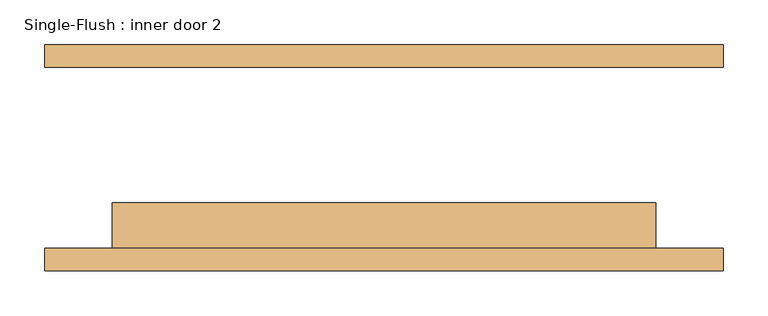
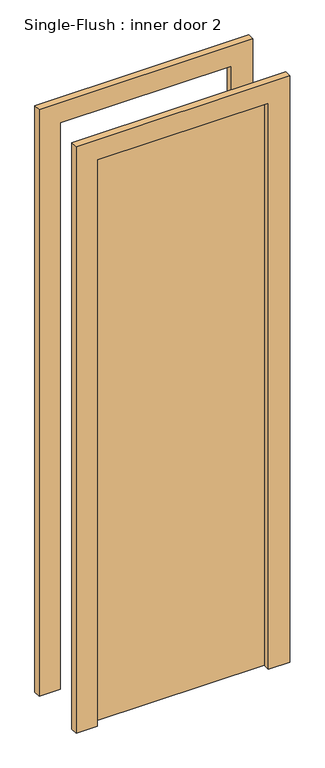
"""IFC4 building model written with IfcOpenShell, lengths in millimetres: door geometry, Single-Flush : inner door 2."""

from ifc_helpers import new_model, si_unit, frame, origin, origin_with_axes, place, context, project, spatial, polyline, outline, extrude, source, transform, mapped, element, save


def single_flush_inner_door_2_1112daf7(model_context):
    return source(origin(), model_context, "Body", "SweptSolid", [
        extrude(outline(polyline([(2209.8, -381.0), (0.0, -381.0), (0.0, -304.8), (2133.6, -304.8), (2133.6, 304.8), (0.0, 304.8), (0.0, 381.0), (2209.8, 381.0), (2209.8, -381.0)])), frame((0.0, -127.0, 0.0), z_axis=(0.0, 1.0, 0.0), x_axis=(0.0, 0.0, 1.0)), (0.0, 0.0, 1.0), 25.4),
        extrude(outline(polyline([(2209.8, 381.0), (2209.8, -381.0), (0.0, -381.0), (0.0, -304.8), (2133.6, -304.8), (2133.6, 304.8), (0.0, 304.8), (0.0, 381.0), (2209.8, 381.0)])), frame((0.0, 101.6, 0.0), z_axis=(0.0, 1.0, 0.0), x_axis=(0.0, 0.0, 1.0)), (0.0, 0.0, 1.0), 25.4),
        extrude(outline(polyline([(304.8, -50.8), (304.8, -101.6), (-304.8, -101.6), (-304.8, -50.8), (304.8, -50.8)])), origin_with_axes(), (0.0, 0.0, 1.0), 2133.6),
    ])


if __name__ == "__main__":
    model = new_model("IFC4")
    model_context = context("Model", 3, world=origin())
    ifc_project = project(units=[si_unit("LENGTHUNIT", "METRE", prefix="MILLI")], contexts=[model_context])
    site = spatial("IfcSite", under=ifc_project)
    building = spatial("IfcBuilding", under=site)
    placement = place(None, origin())
    single_flush_inner_door_2_shape = single_flush_inner_door_2_1112daf7(model_context)
    element("IfcDoor", 1, ObjectType="Single-Flush : inner door 2", at=placement, inside=building, context=model_context, shape_type="MappedRepresentation", body=[
        mapped(single_flush_inner_door_2_shape, transform((0.0, 0.0, 0.0), x_axis=(1.0, 0.0, 0.0), y_axis=(0.0, 1.0, 0.0), z_axis=(0.0, 0.0, 1.0))),
    ])
    save(model, "model.ifc")

# Revit data of these elements
# Type "Single-Flush : inner door 2"
#   Type Mark = "8"
#   Construction Type Id = "MDOOR"
#   Assembly Code = "C1020"
#   Analytic Construction = "Metal"
#   Thickness = 0' - 2"
#   Heat Transfer Coefficient (U) = 0.651978 BTU/(h·ft²·°F)
#   Height = 7' - 0"
#   Trim Projection Ext = 0' - 1"
#   Trim Projection Int = 0' - 1"
#   Trim Width = 0' - 3"
#   Width = 2' - 0"
#   Define Thermal Properties by = 1
#   Door Material = Door - Panel
#   Frame Material = Door - Frame
#   Visual Light Transmittance = 0
#   Solar Heat Gain Coefficient = 0
#   Function = (empty or 0)
#   Wall Closure = (empty or 0)
# Element 1 (IfcDoor, "Single-Flush : inner door 2")
#   Materials on its faces: "Door - Frame", "Door - Panel"
# Materials
#   "Door - Panel": class "Wood", colour RGB 210 159 95, transparency 0
#   "Door - Frame": colour RGB 118 70 51, transparency 0
